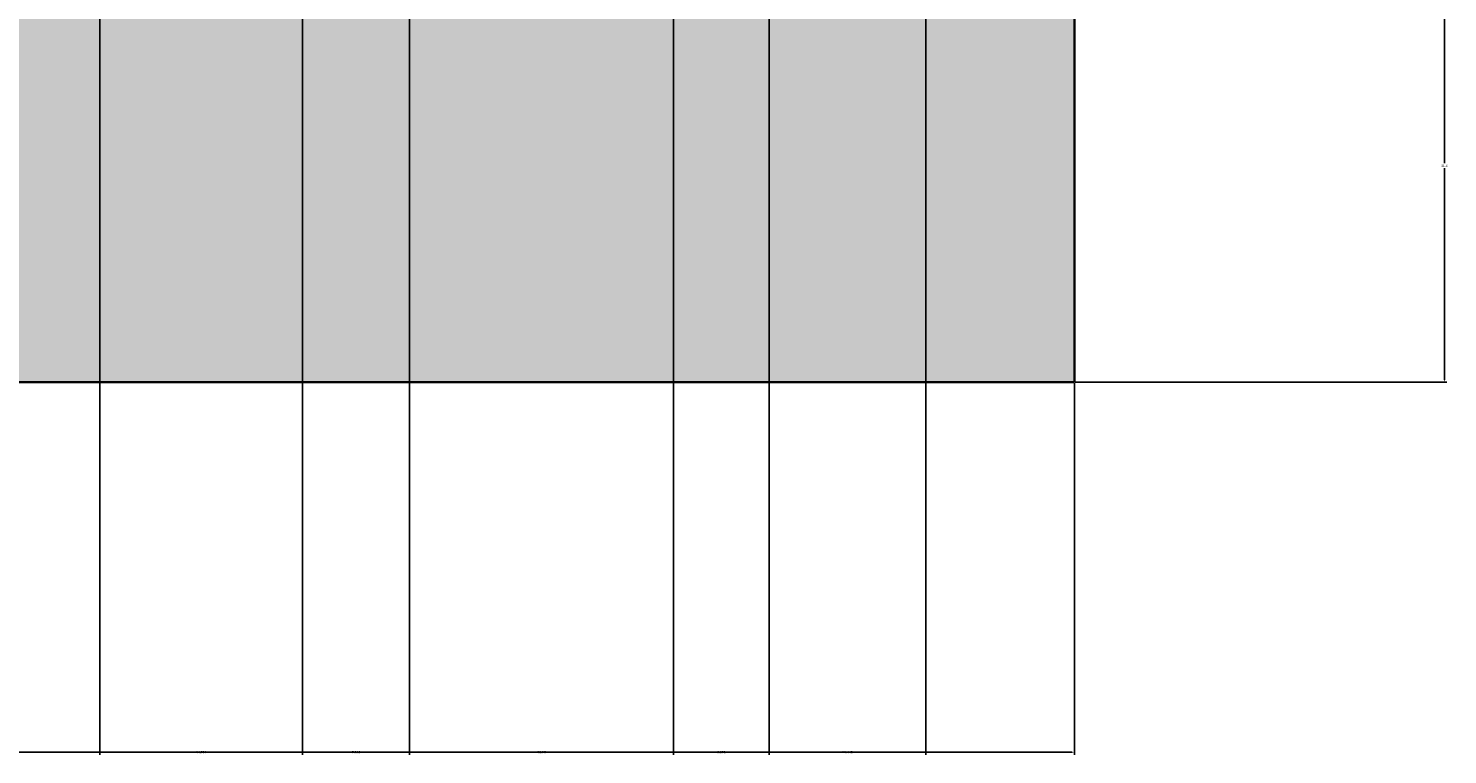
# Model space of a CAD drawing. Units: inches. Extents: x 73 to 607, y 92 to 651.
# Tile 8 of 18: x 504 to 607, y 116 to 169. Entities that reach past the tile are written whole.
import ezdxf

# ---------------------------------------------------------------- set-up
doc = ezdxf.new("R2010")
doc.units = ezdxf.units.IN
doc.header["$MEASUREMENT"] = 0
for name, color, linetype, lineweight in [('A-ANNO-DIMS', 2, 'Continuous', 18), ('A-ELEV', 7, 'Continuous', 35), ('A-ELEV-PATT-BKGD', 252, 'Continuous', 13), ('A-ELEV-PATT-SHAD', 8, 'Continuous', 13)]:
    doc.layers.add(name, color=color, linetype=linetype, lineweight=lineweight)
doc.styles.get("Standard").update_dxf_attribs({"font": 'arial.ttf'})
doc.dimstyles.get("Standard").update_dxf_attribs({"dimtxt": 0.18, "dimasz": 0.18, "dimexe": 0.18, "dimexo": 0.0625, "dimgap": 0.09, "dimtad": 0, "dimtih": 1, "dimtoh": 1, "dimdec": 4, "dimzin": 0, "dimdsep": 46, "dimtxsty": 'Standard', "dimcen": 0.09, "dimadec": 0, "dimazin": 0, "dimtfac": 1, "dimtdec": 4, "dimtofl": 0, "dimtmove": 0, "dimatfit": 3, "dimfxl": 1, "dimtolj": 1, "dimtzin": 0, "dimarcsym": 0})

# ---------------------------------------------------------------- blocks, each defined once
blk = doc.blocks.new('*D4')
at = {"layer": 'A-ANNO-DIMS', "color": 0, "lineweight": -2, "transparency": 16777216}
for p, q in [((100.1, 143.14), (100.1, 116.02)), ((580.1, 143.14), (580.1, 116.02)), ((100.28, 116.2), (339.81, 116.2)), ((579.92, 116.2), (340.39, 116.2))]:
    blk.add_line(p, q, dxfattribs=at)
at = {"layer": 'A-ANNO-DIMS', "color": 0, "transparency": 16777216}
for points in [[(100.28, 116.23), (100.28, 116.17), (100.1, 116.2)], [(579.92, 116.23), (579.92, 116.17), (580.1, 116.2)]]:
    blk.add_solid(points, dxfattribs=at)
at = {"layer": 'Defpoints', "color": 0, "transparency": 16777216}
for p in [(100.1, 143.2), (580.1, 143.2), (580.1, 116.2)]:
    blk.add_point(p, dxfattribs=at)
at = {"layer": 'A-ANNO-DIMS', "color": 0, "transparency": 16777216, "insert": (340.1, 116.2), "char_height": 0.18, "attachment_point": 5}
blk.add_mtext('\\A1;480', dxfattribs=at)
blk = doc.blocks.new('*D15')
at = {"layer": 'A-ANNO-DIMS', "color": 0, "lineweight": -2, "transparency": 16777216}
for p, q in [((454.77, 174.8), (607.28, 174.8)), ((607.1, 174.62), (607.1, 159.19)), ((607.1, 143.38), (607.1, 158.82)), ((580.16, 143.2), (607.28, 143.2))]:
    blk.add_line(p, q, dxfattribs=at)
at = {"layer": 'A-ANNO-DIMS', "color": 0, "transparency": 16777216}
for points in [[(607.07, 174.62), (607.13, 174.62), (607.1, 174.8)], [(607.07, 143.38), (607.13, 143.38), (607.1, 143.2)]]:
    blk.add_solid(points, dxfattribs=at)
at = {"layer": 'Defpoints', "color": 0, "transparency": 16777216}
for p in [(454.7, 174.8), (607.1, 174.8), (580.1, 143.2)]:
    blk.add_point(p, dxfattribs=at)
at = {"layer": 'A-ANNO-DIMS', "color": 0, "transparency": 16777216, "insert": (607.1, 159), "char_height": 0.18, "attachment_point": 5}
blk.add_mtext('\\A1;31.6', dxfattribs=at)
blk = doc.blocks.new('*D113')
at = {"layer": 'A-ANNO-DIMS', "color": 0, "lineweight": -2, "transparency": 16777216}
for p, q in [((508.96, 194.7), (508.96, 116.02)), ((492.77, 181.6), (492.77, 116.02)), ((492.95, 116.2), (500.48, 116.2)), ((508.78, 116.2), (501.25, 116.2))]:
    blk.add_line(p, q, dxfattribs=at)
at = {"layer": 'A-ANNO-DIMS', "color": 0, "transparency": 16777216}
for points in [[(492.95, 116.23), (492.95, 116.17), (492.77, 116.2)], [(508.78, 116.23), (508.78, 116.17), (508.96, 116.2)]]:
    blk.add_solid(points, dxfattribs=at)
at = {"layer": 'Defpoints', "color": 0, "transparency": 16777216}
for p in [(508.96, 194.77), (492.77, 181.66), (508.96, 116.2)]:
    blk.add_point(p, dxfattribs=at)
at = {"layer": 'A-ANNO-DIMS', "color": 0, "transparency": 16777216, "insert": (500.86, 116.2), "char_height": 0.18, "attachment_point": 5}
blk.add_mtext('\\A1;16.19', dxfattribs=at)
blk = doc.blocks.new('*D114')
at = {"layer": 'A-ANNO-DIMS', "color": 0, "lineweight": -2, "transparency": 16777216}
for p, q in [((508.96, 194.7), (508.96, 116.02)), ((523.75, 186.62), (523.75, 116.02)), ((509.14, 116.2), (515.9, 116.2)), ((523.57, 116.2), (516.81, 116.2))]:
    blk.add_line(p, q, dxfattribs=at)
at = {"layer": 'A-ANNO-DIMS', "color": 0, "transparency": 16777216}
for points in [[(509.14, 116.23), (509.14, 116.17), (508.96, 116.2)], [(523.57, 116.23), (523.57, 116.17), (523.75, 116.2)]]:
    blk.add_solid(points, dxfattribs=at)
at = {"layer": 'Defpoints', "color": 0, "transparency": 16777216}
for p in [(508.96, 194.77), (523.75, 186.68), (523.75, 116.2)]:
    blk.add_point(p, dxfattribs=at)
at = {"layer": 'A-ANNO-DIMS', "color": 0, "transparency": 16777216, "insert": (516.36, 116.2), "char_height": 0.18, "attachment_point": 5}
blk.add_mtext('\\A1;14.794', dxfattribs=at)
blk = doc.blocks.new('*D115')
at = {"layer": 'A-ANNO-DIMS', "color": 0, "lineweight": -2, "transparency": 16777216}
for p, q in [((531.57, 203.63), (531.57, 116.02)), ((523.75, 186.62), (523.75, 116.02)), ((523.93, 116.2), (527.27, 116.2)), ((531.39, 116.2), (528.05, 116.2))]:
    blk.add_line(p, q, dxfattribs=at)
at = {"layer": 'A-ANNO-DIMS', "color": 0, "transparency": 16777216}
for points in [[(523.93, 116.23), (523.93, 116.17), (523.75, 116.2)], [(531.39, 116.23), (531.39, 116.17), (531.57, 116.2)]]:
    blk.add_solid(points, dxfattribs=at)
at = {"layer": 'Defpoints', "color": 0, "transparency": 16777216}
for p in [(531.57, 203.69), (523.75, 186.68), (531.57, 116.2)]:
    blk.add_point(p, dxfattribs=at)
at = {"layer": 'A-ANNO-DIMS', "color": 0, "transparency": 16777216, "insert": (527.66, 116.2), "char_height": 0.18, "attachment_point": 5}
blk.add_mtext('\\A1;7.816', dxfattribs=at)
blk = doc.blocks.new('*D116')
at = {"layer": 'A-ANNO-DIMS', "color": 0, "lineweight": -2, "transparency": 16777216}
for p, q in [((531.57, 203.63), (531.57, 116.02)), ((550.83, 183.55), (550.83, 116.02)), ((531.75, 116.2), (540.81, 116.2)), ((550.65, 116.2), (541.58, 116.2))]:
    blk.add_line(p, q, dxfattribs=at)
at = {"layer": 'A-ANNO-DIMS', "color": 0, "transparency": 16777216}
for points in [[(531.75, 116.23), (531.75, 116.17), (531.57, 116.2)], [(550.65, 116.23), (550.65, 116.17), (550.83, 116.2)]]:
    blk.add_solid(points, dxfattribs=at)
at = {"layer": 'Defpoints', "color": 0, "transparency": 16777216}
for p in [(531.57, 203.69), (550.83, 183.61), (550.83, 116.2)]:
    blk.add_point(p, dxfattribs=at)
at = {"layer": 'A-ANNO-DIMS', "color": 0, "transparency": 16777216, "insert": (541.2, 116.2), "char_height": 0.18, "attachment_point": 5}
blk.add_mtext('\\A1;19.26', dxfattribs=at)
blk = doc.blocks.new('*D117')
at = {"layer": 'A-ANNO-DIMS', "color": 0, "lineweight": -2, "transparency": 16777216}
for p, q in [((557.81, 203.91), (557.81, 116.02)), ((550.83, 183.55), (550.83, 116.02)), ((551.01, 116.2), (553.92, 116.2)), ((557.63, 116.2), (554.71, 116.2))]:
    blk.add_line(p, q, dxfattribs=at)
at = {"layer": 'A-ANNO-DIMS', "color": 0, "transparency": 16777216}
for points in [[(551.01, 116.23), (551.01, 116.17), (550.83, 116.2)], [(557.63, 116.23), (557.63, 116.17), (557.81, 116.2)]]:
    blk.add_solid(points, dxfattribs=at)
at = {"layer": 'Defpoints', "color": 0, "transparency": 16777216}
for p in [(557.81, 203.97), (550.83, 183.61), (557.81, 116.2)]:
    blk.add_point(p, dxfattribs=at)
at = {"layer": 'A-ANNO-DIMS', "color": 0, "transparency": 16777216, "insert": (554.32, 116.2), "char_height": 0.18, "attachment_point": 5}
blk.add_mtext('\\A1;6.978', dxfattribs=at)
blk = doc.blocks.new('*D118')
at = {"layer": 'A-ANNO-DIMS', "color": 0, "lineweight": -2, "transparency": 16777216}
for p, q in [((557.81, 203.91), (557.81, 116.02)), ((569.25, 193.31), (569.25, 116.02)), ((557.99, 116.2), (563.07, 116.2)), ((569.07, 116.2), (563.99, 116.2))]:
    blk.add_line(p, q, dxfattribs=at)
at = {"layer": 'A-ANNO-DIMS', "color": 0, "transparency": 16777216}
for points in [[(557.99, 116.23), (557.99, 116.17), (557.81, 116.2)], [(569.07, 116.23), (569.07, 116.17), (569.25, 116.2)]]:
    blk.add_solid(points, dxfattribs=at)
at = {"layer": 'Defpoints', "color": 0, "transparency": 16777216}
for p in [(557.81, 203.97), (569.25, 193.37), (569.25, 116.2)]:
    blk.add_point(p, dxfattribs=at)
at = {"layer": 'A-ANNO-DIMS', "color": 0, "transparency": 16777216, "insert": (563.53, 116.2), "char_height": 0.18, "attachment_point": 5}
blk.add_mtext('\\A1;11.445', dxfattribs=at)

msp = doc.modelspace()

# ---------------------------------------------------------------- hatches: boundary and pattern name
at = {"layer": 'A-ELEV-PATT-BKGD'}
h = msp.add_hatch(color=256, dxfattribs=at)
h.dxf.hatch_style = 1
h.paths.add_polyline_path([(321.3008, 479.2042), (312.3008, 479.2042), (312.3008, 478.7576), (312.3008, 412.636), (321.3008, 412.636)])
h.paths.add_polyline_path([(312.3008, 504.7576), (256.4726, 504.7576), (256.4726, 503.4576), (312.3008, 503.4576)], flags=17)
h.paths.add_polyline_path([(321.3008, 543.1576), (321.3008, 552.1576), (320.3257, 552.1576), (312.3008, 552.1576), (256.4726, 552.1576), (256.4726, 543.1576), (312.3008, 543.1576), (312.3008, 479.2042), (321.3008, 479.2042)])
h.paths.add_polyline_path([(451.5214, 412.636), (256.4726, 412.636), (256.4726, 403.636), (442.5214, 403.636), (442.5214, 320.2042), (206.1343, 320.2042), (206.1343, 320.9135), (206.1343, 403.636), (256.4726, 403.636), (256.4726, 412.636), (201.6343, 412.636), (201.6343, 320.9135), (201.6343, 320.2042), (201.6343, 311.2042), (256.4726, 311.2042), (451.5214, 311.2042)])
h.paths.add_polyline_path([(431.07, 258.6914), (369.5339, 258.6914), (369.5339, 247.4054), (396.692, 247.4054), (425.07, 247.4054), (425.07, 194.7312), (396.692, 194.6197), (396.692, 194.5366), (369.5339, 194.5366), (369.5339, 185.6619), (431.07, 185.6619)])
h.paths.add_polyline_path([(580.0983, 262.3024), (451.5214, 262.3024), (451.5214, 143.2042), (580.0983, 143.2042)])
h.paths.add_polyline_path([(454.7049, 174.802), (454.7049, 256.6321), (577.9249, 256.6321), (577.9249, 174.802)], flags=16)
h.paths.add_polyline_path([(465.9716, 191.1416, -1), (473.7874, 191.1416, -1)], flags=0)
h.paths.add_polyline_path([(490.5373, 181.6586, -1), (494.9999, 181.6586, -1)], flags=0)
h.paths.add_polyline_path([(476.2996, 209.8287, -1), (500.5844, 209.8287, -1)], flags=0)
h.paths.add_polyline_path([(505.3326, 194.7675, -1), (512.5843, 194.7675, -1)], flags=0)
h.paths.add_polyline_path([(520.9613, 186.679, -1), (526.544, 186.679, -1)], flags=0)
h.paths.add_polyline_path([(466.8103, 225.7267, -1), (470.1573, 225.7267, -1)], flags=0)
h.paths.add_polyline_path([(527.1059, 203.6926, -1), (536.0311, 203.6926, -1)], flags=0)
h.paths.add_polyline_path([(504.775, 232.6995, -1), (513.7002, 232.6995, -1)], flags=0)
h.paths.add_polyline_path([(546.9241, 183.611, -1), (554.7336, 183.611, -1)], flags=0)
h.paths.add_polyline_path([(459.5544, 243.856, -1), (466.8061, 243.856, -1)], flags=0)
h.paths.add_polyline_path([(476.3045, 246.924, -1), (488.5767, 246.924, -1)], flags=0)
h.paths.add_polyline_path([(529.9044, 226.8424, -1), (556.68, 226.8424, -1)], flags=0)
h.paths.add_polyline_path([(554.1814, 203.9716, -1), (561.4331, 203.9716, -1)], flags=0)
h.paths.add_polyline_path([(567.8561, 193.3729, -1), (570.6475, 193.3729, -1)], flags=0)
h.paths.add_polyline_path([(522.3584, 250.271, -1), (525.7053, 250.271, -1)], flags=0)
h.paths.add_polyline_path([(561.9965, 245.2506, -1), (567.5748, 245.2506, -1)], flags=0)
h.paths.add_polyline_path([(347.8686, 194.5366), (341.8686, 194.5366), (341.8686, 194.5452), (314.0144, 194.5452), (314.0144, 188.5452), (347.8686, 188.5452)])
h.paths.add_polyline_path([(347.8686, 253.4054), (314.0144, 253.4054), (314.0144, 247.4054), (341.8686, 247.4054), (347.8686, 247.4054)])
h.paths.add_polyline_path([(304.3559, 253.4054), (298.3559, 253.4054), (298.3559, 188.5452), (304.3559, 188.5452)])
h.paths.add_polyline_path([(450.6603, 552.1576), (369.9727, 552.1576), (369.9727, 479.2042), (374.4727, 479.2042), (374.4727, 547.6576), (446.1603, 547.6576), (446.1603, 479.2042), (450.6603, 479.2042)])
h.paths.add_polyline_path([(374.4727, 479.2042), (369.9727, 479.2042), (369.9727, 465.0632), (374.4727, 465.0632)])
h.paths.add_polyline_path([(450.6603, 479.2042), (446.1603, 479.2042), (446.1603, 465.0632), (450.6603, 465.0632)])
h.paths.add_polyline_path([(256.4726, 281.6039), (109.0983, 281.6039), (100.0983, 281.6039), (100.0983, 167.2042), (100.0983, 143.2042), (109.0983, 143.2042), (109.0983, 167.2042), (109.0983, 272.6039), (256.4726, 272.6039)])
at = {"layer": 'A-ELEV-PATT-SHAD'}
h = msp.add_hatch(color=256, dxfattribs=at)
h.dxf.hatch_style = 1
h.paths.add_polyline_path([(451.5214, 412.636), (256.4726, 412.636), (256.4726, 403.636), (442.5214, 403.636), (442.5214, 320.2042), (206.1343, 320.2042), (206.1343, 320.9135), (206.1343, 403.636), (256.4726, 403.636), (256.4726, 412.636), (201.6343, 412.636), (201.6343, 320.9135), (201.6343, 320.2042), (201.6343, 311.2042), (256.4726, 311.2042), (451.5214, 311.2042)])
h.paths.add_polyline_path([(580.0983, 262.3024), (451.5214, 262.3024), (451.5214, 143.2042), (580.0983, 143.2042)])
h.paths.add_polyline_path([(454.7049, 174.802), (454.7049, 256.6321), (577.9249, 256.6321), (577.9249, 174.802)], flags=16)
h.paths.add_polyline_path([(465.9716, 191.1416, -1), (473.7874, 191.1416, -1)], flags=0)
h.paths.add_polyline_path([(490.5373, 181.6586, -1), (494.9999, 181.6586, -1)], flags=0)
h.paths.add_polyline_path([(476.2996, 209.8287, -1), (500.5844, 209.8287, -1)], flags=0)
h.paths.add_polyline_path([(505.3326, 194.7675, -1), (512.5843, 194.7675, -1)], flags=0)
h.paths.add_polyline_path([(520.9613, 186.679, -1), (526.544, 186.679, -1)], flags=0)
h.paths.add_polyline_path([(466.8103, 225.7267, -1), (470.1573, 225.7267, -1)], flags=0)
h.paths.add_polyline_path([(527.1059, 203.6926, -1), (536.0311, 203.6926, -1)], flags=0)
h.paths.add_polyline_path([(459.5544, 243.856, -1), (466.8061, 243.856, -1)], flags=0)
h.paths.add_polyline_path([(504.775, 232.6995, -1), (513.7002, 232.6995, -1)], flags=0)
h.paths.add_polyline_path([(476.3045, 246.924, -1), (488.5767, 246.924, -1)], flags=0)
h.paths.add_polyline_path([(546.9241, 183.611, -1), (554.7336, 183.611, -1)], flags=0)
h.paths.add_polyline_path([(529.9044, 226.8424, -1), (556.68, 226.8424, -1)], flags=0)
h.paths.add_polyline_path([(554.1814, 203.9716, -1), (561.4331, 203.9716, -1)], flags=0)
h.paths.add_polyline_path([(522.3584, 250.271, -1), (525.7053, 250.271, -1)], flags=0)
h.paths.add_polyline_path([(567.8561, 193.3729, -1), (570.6475, 193.3729, -1)], flags=0)
h.paths.add_polyline_path([(561.9965, 245.2506, -1), (567.5748, 245.2506, -1)], flags=0)
h.paths.add_polyline_path([(431.07, 258.6914), (369.5339, 258.6914), (369.5339, 247.4054), (396.692, 247.4054), (425.07, 247.4054), (425.07, 194.7312), (396.692, 194.6197), (396.692, 194.5366), (369.5339, 194.5366), (369.5339, 185.6619), (431.07, 185.6619)])
h.paths.add_polyline_path([(347.8686, 253.4054), (314.0144, 253.4054), (314.0144, 247.4054), (341.8686, 247.4054), (347.8686, 247.4054)])
h.paths.add_polyline_path([(304.3559, 253.4054), (298.3559, 253.4054), (298.3559, 188.5452), (304.3559, 188.5452)])
h.paths.add_polyline_path([(347.8686, 194.5366), (341.8686, 194.5366), (341.8686, 194.5452), (314.0144, 194.5452), (314.0144, 188.5452), (347.8686, 188.5452)])

# ---------------------------------------------------------------- linework, layer by layer
at = {"layer": 'A-ELEV'}
for p, q in [((580.0983, 167.2042), (580.0983, 311.2042)), ((580.0983, 143.2042), (580.0983, 167.2042)), ((100.0983, 143.2042), (580.0983, 143.2042))]:
    msp.add_line(p, q, dxfattribs=at)
msp.add_lwpolyline([(580.0983, 143.2042), (451.5214, 143.2042), (451.5214, 262.3024), (580.0983, 262.3024)], close=True, dxfattribs=at)

# ---------------------------------------------------------------- dimensions: what is measured, and where the dimension line sits
at = {"layer": 'A-ANNO-DIMS'}
for base, p1, p2, override, picture, middle in [((531.5685, 116.2042), (523.7527, 186.679), (531.5685, 203.6926), {"dimdec": 3, "dimlfac": 1, "dimrnd": 0, "dimzin": 0, "dimdsep": 46, "dimlunit": 2}, '*D115', (527.6606, 116.2042)), ((550.8289, 116.2042), (531.5685, 203.6926), (550.8289, 183.611), {"dimdec": 2, "dimlfac": 1, "dimrnd": 0, "dimzin": 0, "dimdsep": 46, "dimlunit": 2}, '*D116', (541.1987, 116.2042)), ((557.8072, 116.2042), (550.8289, 183.611), (557.8072, 203.9716), {"dimdec": 3, "dimlfac": 1, "dimrnd": 0, "dimzin": 0, "dimdsep": 46, "dimlunit": 2}, '*D117', (554.3181, 116.2042)), ((569.2518, 116.2042), (557.8072, 203.9716), (569.2518, 193.3729), {"dimdec": 3, "dimlfac": 1, "dimrnd": 0, "dimzin": 0, "dimdsep": 46, "dimlunit": 2}, '*D118', (563.5295, 116.2042)), ((508.9585, 116.2042), (492.7686, 181.6586), (508.9585, 194.7675), {"dimdec": 2, "dimlfac": 1, "dimrnd": 0, "dimzin": 0, "dimdsep": 46, "dimlunit": 2}, '*D113', (500.8636, 116.2042)), ((523.7527, 116.2042), (508.9585, 194.7675), (523.7527, 186.679), {"dimdec": 3, "dimlfac": 1, "dimrnd": 0, "dimzin": 0, "dimdsep": 46, "dimlunit": 2}, '*D114', (516.3556, 116.2042)), ((580.0983, 116.2042), (100.0983, 143.2042), (580.0983, 143.2042), {"dimdec": 0, "dimlfac": 1, "dimrnd": 0, "dimzin": 0, "dimdsep": 46, "dimlunit": 2}, '*D4', (340.0983, 116.2042))]:
    dim = msp.add_linear_dim(base=base, p1=p1, p2=p2, dimstyle='Standard', override=override, dxfattribs=at)
    dim.commit()
    dim.dimension.update_dxf_attribs({"geometry": picture, "text_midpoint": middle})
dim = msp.add_linear_dim(base=(607.0983, 174.802), p1=(580.0983, 143.2042), p2=(454.7049, 174.802), angle=90, dimstyle='Standard', override={"dimdec": 1, "dimlfac": 1, "dimrnd": 0, "dimzin": 0, "dimdsep": 46, "dimlunit": 2}, dxfattribs=at)
dim.commit()
dim.dimension.update_dxf_attribs({"geometry": '*D15', "text_midpoint": (607.0983, 159.0031)})

doc.saveas('drawing.dxf')
